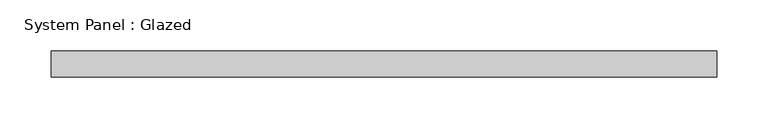
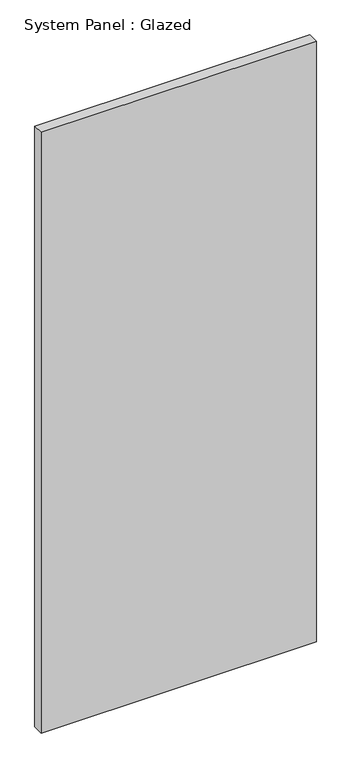
"""IFC4 building model written with IfcOpenShell, lengths in millimetres: plate geometry, System Panel : Glazed."""

from ifc_helpers import new_model, si_unit, origin, origin_with_axes, place, context, project, spatial, polyline, outline, extrude, source, transform, mapped, element, save


def system_panel_glazed_6adbe530(model_context):
    return source(origin(), model_context, "Body", "SweptSolid", [
        extrude(outline(polyline([(323.85, 19.05), (-323.85, 19.05), (-323.85, 44.45), (323.85, 44.45), (323.85, 19.05)])), origin_with_axes(), (0.0, 0.0, 1.0), 1493.8138027),
    ])


if __name__ == "__main__":
    model = new_model("IFC4")
    model_context = context("Model", 3, world=origin())
    ifc_project = project(units=[si_unit("LENGTHUNIT", "METRE", prefix="MILLI")], contexts=[model_context])
    site = spatial("IfcSite", under=ifc_project)
    building = spatial("IfcBuilding", under=site)
    placement = place(None, origin())
    system_panel_glazed_shape = system_panel_glazed_6adbe530(model_context)
    element("IfcPlate", 1, ObjectType="System Panel : Glazed", at=placement, inside=building, context=model_context, shape_type="MappedRepresentation", body=[
        mapped(system_panel_glazed_shape, transform((0.0, 0.0, 0.0), x_axis=(1.0, 0.0, 0.0), y_axis=(0.0, 1.0, 0.0), z_axis=(0.0, 0.0, 1.0))),
    ])
    save(model, "model.ifc")

# Revit data of these elements
# Type "System Panel : Glazed"
#   Construction Type Id = "GSP4R"
#   Analytic Construction = "1/8 in Pilkington single glazing"
#   Visual Light Transmittance = 0.9
#   Solar Heat Gain Coefficient = 0.86
#   Heat Transfer Coefficient (U) = 1.18115 BTU/(h·ft²·°F)
#   Define Thermal Properties by = 1
# Element 1 (IfcPlate, "System Panel : Glazed")
#   Materials on its faces: "Glass"
# Materials
#   "Glass": class "Glass", colour RGB 0 128 192, transparency 0.75, Description = "Soda Lime Glass", Cost = 0
